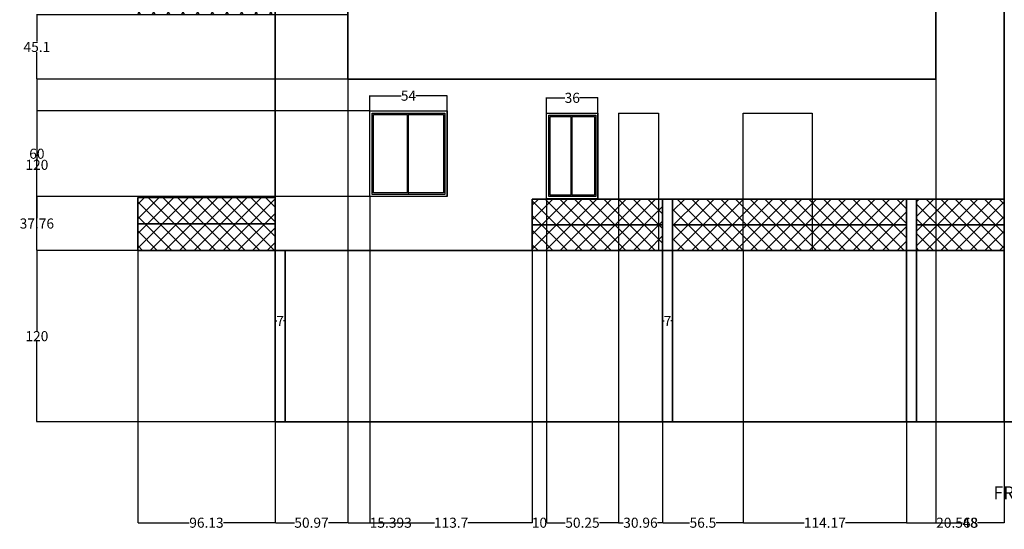
# Model space of a CAD drawing. Units: inches. Extents: x -222 to 1347, y 12 to 1073.
# Tile 1 of 4: x -222 to 467, y 12 to 369. Entities that reach past the tile are written whole.
import ezdxf

# ---------------------------------------------------------------- set-up
doc = ezdxf.new("R2010")
doc.units = ezdxf.units.IN
doc.header["$MEASUREMENT"] = 0
for name, color, linetype, lineweight in [('A-ANNO-DIMS', 2, 'Continuous', 18), ('A-ANNO-TEXT', 7, 'Continuous', 25), ('A-DOOR', 4, 'Continuous', 25), ('A-ELEV', 7, 'Continuous', 35), ('A-ELEV-PATT', 8, 'Continuous', 13), ('A-GLAZ', 4, 'Continuous', 25)]:
    doc.layers.add(name, color=color, linetype=linetype, lineweight=lineweight)
doc.styles.get("Standard").update_dxf_attribs({"font": 'arial.ttf'})
doc.dimstyles.get("Standard").update_dxf_attribs({"dimtxt": 7.0625, "dimasz": 0.18, "dimexe": 0.18, "dimexo": 0.0625, "dimgap": 0.09, "dimtad": 0, "dimtih": 1, "dimtoh": 1, "dimdec": 4, "dimzin": 0, "dimdsep": 46, "dimlunit": 4, "dimtxsty": 'Standard', "dimcen": 0.09, "dimadec": 0, "dimazin": 0, "dimtfac": 1, "dimtdec": 4, "dimtofl": 0, "dimtmove": 0, "dimatfit": 3, "dimfxl": 1, "dimtolj": 1, "dimtzin": 0, "dimarcsym": 0})

# ---------------------------------------------------------------- blocks, each defined once
blk = doc.blocks.new('*U2')
for p, q in [((1.5, 1.5), (1.5, 58.5)), ((1.5, 58.5), (27, 58.5)), ((27, 1.5), (27, 58.5)), ((27, 58.5), (52.5, 58.5)), ((52.5, 58.5), (52.5, 1.5)), ((27, 1.5), (1.5, 1.5)), ((52.5, 1.5), (27, 1.5))]:
    blk.add_line(p, q)
blk.add_lwpolyline([(0, 0), (0, 60), (54, 60), (54, 0)], close=True)
for points in [[(26, 57.5), (26, 2.5), (2.5, 2.5), (2.5, 57.5), (26, 57.5)], [(27, 57.5), (51.5, 57.5), (51.5, 2.5), (27, 2.5)]]:
    blk.add_lwpolyline(points)
blk = doc.blocks.new('*U3')
for p, q in [((1.5, 1.5), (1.5, 58.5)), ((1.5, 58.5), (18, 58.5)), ((18, 1.5), (18, 58.5)), ((18, 58.5), (34.5, 58.5)), ((34.5, 58.5), (34.5, 1.5)), ((18, 1.5), (1.5, 1.5)), ((34.5, 1.5), (18, 1.5))]:
    blk.add_line(p, q)
blk.add_lwpolyline([(0, 0), (0, 60), (36, 60), (36, 0)], close=True)
for points in [[(17, 57.5), (17, 2.5), (2.5, 2.5), (2.5, 57.5), (17, 57.5)], [(18, 57.5), (33.5, 57.5), (33.5, 2.5), (18, 2.5)]]:
    blk.add_lwpolyline(points)
blk = doc.blocks.new('DOOR-700')
for p, q in [((0, 96.26), (0, 0)), ((0, 96.26), (23.43, 96.26)), ((23.43, 96.26), (28.14, 96.26)), ((28.14, 96.26), (28.14, 0))]:
    blk.add_line(p, q)
blk = doc.blocks.new('DOOR-1200')
for p, q in [((0, 0), (0, 96.26)), ((0, 96.26), (48.21, 96.26)), ((48.21, 96.26), (48.21, 0))]:
    blk.add_line(p, q)
blk = doc.blocks.new('*D11')
at = {"layer": 'A-ANNO-DIMS', "color": 0, "lineweight": -2, "transparency": 16777216}
for p, q in [((-139.29, 207.6), (-139.29, 16.83)), ((-43.16, 87.6), (-43.16, 16.83)), ((-139.11, 17.01), (-103.23, 17.01)), ((-43.34, 17.01), (-79.22, 17.01))]:
    blk.add_line(p, q, dxfattribs=at)
at = {"layer": 'A-ANNO-DIMS', "color": 0, "transparency": 16777216}
for points in [[(-139.11, 17.04), (-139.11, 16.98), (-139.29, 17.01)], [(-43.34, 17.04), (-43.34, 16.98), (-43.16, 17.01)]]:
    blk.add_solid(points, dxfattribs=at)
at = {"layer": 'Defpoints', "color": 0, "transparency": 16777216}
for p in [(-139.29, 207.66), (-43.16, 87.66), (-43.16, 17.01)]:
    blk.add_point(p, dxfattribs=at)
at = {"layer": 'A-ANNO-DIMS', "color": 0, "transparency": 16777216, "insert": (-91.23, 17.01), "char_height": 7.062, "attachment_point": 5}
blk.add_mtext('\\A1;96.13', dxfattribs=at)
blk = doc.blocks.new('*D12')
at = {"layer": 'A-ANNO-DIMS', "color": 0, "lineweight": -2, "transparency": 16777216}
for p, q in [((7.81, 327.6), (7.81, 16.83)), ((-43.16, 87.6), (-43.16, 16.83)), ((-42.98, 17.01), (-29.68, 17.01)), ((7.63, 17.01), (-5.67, 17.01))]:
    blk.add_line(p, q, dxfattribs=at)
at = {"layer": 'A-ANNO-DIMS', "color": 0, "transparency": 16777216}
for points in [[(-42.98, 17.04), (-42.98, 16.98), (-43.16, 17.01)], [(7.63, 17.04), (7.63, 16.98), (7.81, 17.01)]]:
    blk.add_solid(points, dxfattribs=at)
at = {"layer": 'Defpoints', "color": 0, "transparency": 16777216}
for p in [(7.81, 327.66), (-43.16, 87.66), (7.81, 17.01)]:
    blk.add_point(p, dxfattribs=at)
at = {"layer": 'A-ANNO-DIMS', "color": 0, "transparency": 16777216, "insert": (-17.68, 17.01), "char_height": 7.062, "attachment_point": 5}
blk.add_mtext('\\A1;50.97', dxfattribs=at)
blk = doc.blocks.new('*D13')
at = {"layer": 'A-ANNO-DIMS', "color": 0, "lineweight": -2, "transparency": 16777216}
for p, q in [((7.81, 327.6), (7.81, 16.83)), ((23.2, 245.36), (23.2, 16.83)), ((7.99, 17.01), (23.02, 17.01)), ((23.2, 17.01), (23.38, 17.01))]:
    blk.add_line(p, q, dxfattribs=at)
at = {"layer": 'A-ANNO-DIMS', "color": 0, "transparency": 16777216}
for points in [[(7.99, 17.04), (7.99, 16.98), (7.81, 17.01)], [(23.02, 17.04), (23.02, 16.98), (23.2, 17.01)]]:
    blk.add_solid(points, dxfattribs=at)
at = {"layer": 'Defpoints', "color": 0, "transparency": 16777216}
for p in [(7.81, 327.66), (23.2, 245.43), (23.2, 17.01)]:
    blk.add_point(p, dxfattribs=at)
at = {"layer": 'A-ANNO-DIMS', "color": 0, "transparency": 16777216, "insert": (37.8, 17.01), "char_height": 7.062, "attachment_point": 5}
blk.add_mtext('\\A1;15.393', dxfattribs=at)
blk = doc.blocks.new('*D14')
at = {"layer": 'A-ANNO-DIMS', "color": 0, "lineweight": -2, "transparency": 16777216}
for p, q in [((23.2, 245.36), (23.2, 16.83)), ((136.89, 207.6), (136.89, 16.83)), ((23.38, 17.01), (68.37, 17.01)), ((136.71, 17.01), (91.72, 17.01))]:
    blk.add_line(p, q, dxfattribs=at)
at = {"layer": 'A-ANNO-DIMS', "color": 0, "transparency": 16777216}
for points in [[(23.38, 17.04), (23.38, 16.98), (23.2, 17.01)], [(136.71, 17.04), (136.71, 16.98), (136.89, 17.01)]]:
    blk.add_solid(points, dxfattribs=at)
at = {"layer": 'Defpoints', "color": 0, "transparency": 16777216}
for p in [(23.2, 245.43), (136.89, 207.66), (136.89, 17.01)]:
    blk.add_point(p, dxfattribs=at)
at = {"layer": 'A-ANNO-DIMS', "color": 0, "transparency": 16777216, "insert": (80.04, 17.01), "char_height": 7.062, "attachment_point": 5}
blk.add_mtext('\\A1;113.7', dxfattribs=at)
blk = doc.blocks.new('*D15')
at = {"layer": 'A-ANNO-DIMS', "color": 0, "lineweight": -2, "transparency": 16777216}
for p, q in [((146.891371, 243.863959), (146.891371, 16.834205)), ((136.890751, 207.601705), (136.890751, 16.834205)), ((136.710751, 17.014205), (136.530751, 17.014205)), ((147.071371, 17.014205), (147.251371, 17.014205))]:
    blk.add_line(p, q, dxfattribs=at)
at = {"layer": 'A-ANNO-DIMS', "color": 0, "transparency": 16777216}
for points in [[(136.710751, 17.044205), (136.710751, 16.984205), (136.890751, 17.014205)], [(147.071371, 17.044205), (147.071371, 16.984205), (146.891371, 17.014205)]]:
    blk.add_solid(points, dxfattribs=at)
at = {"layer": 'Defpoints', "color": 0, "transparency": 16777216}
for p in [(146.891371, 243.926459), (136.890751, 207.664205), (146.891371, 17.014205)]:
    blk.add_point(p, dxfattribs=at)
at = {"layer": 'A-ANNO-DIMS', "color": 0, "transparency": 16777216, "insert": (141.891061, 17.014205), "char_height": 7.0625, "attachment_point": 5}
blk.add_mtext('\\A1;10', dxfattribs=at)
blk = doc.blocks.new('*D16')
at = {"layer": 'A-ANNO-DIMS', "color": 0, "lineweight": -2, "transparency": 16777216}
for p, q in [((146.89, 243.86), (146.89, 16.83)), ((197.14, 207.6), (197.14, 16.83)), ((147.07, 17.01), (159.98, 17.01)), ((196.96, 17.01), (184.05, 17.01))]:
    blk.add_line(p, q, dxfattribs=at)
at = {"layer": 'A-ANNO-DIMS', "color": 0, "transparency": 16777216}
for points in [[(147.07, 17.04), (147.07, 16.98), (146.89, 17.01)], [(196.96, 17.04), (196.96, 16.98), (197.14, 17.01)]]:
    blk.add_solid(points, dxfattribs=at)
at = {"layer": 'Defpoints', "color": 0, "transparency": 16777216}
for p in [(146.89, 243.93), (197.14, 207.66), (197.14, 17.01)]:
    blk.add_point(p, dxfattribs=at)
at = {"layer": 'A-ANNO-DIMS', "color": 0, "transparency": 16777216, "insert": (172.02, 17.01), "char_height": 7.062, "attachment_point": 5}
blk.add_mtext('\\A1;50.25', dxfattribs=at)
blk = doc.blocks.new('*D17')
at = {"layer": 'A-ANNO-DIMS', "color": 0, "lineweight": -2, "transparency": 16777216}
for p, q in [((197.14, 207.6), (197.14, 16.83)), ((228.1, 87.6), (228.1, 16.83)), ((197.32, 17.01), (200.62, 17.01)), ((227.92, 17.01), (224.62, 17.01))]:
    blk.add_line(p, q, dxfattribs=at)
at = {"layer": 'A-ANNO-DIMS', "color": 0, "transparency": 16777216}
for points in [[(197.32, 17.04), (197.32, 16.98), (197.14, 17.01)], [(227.92, 17.04), (227.92, 16.98), (228.1, 17.01)]]:
    blk.add_solid(points, dxfattribs=at)
at = {"layer": 'Defpoints', "color": 0, "transparency": 16777216}
for p in [(197.14, 207.66), (228.1, 87.66), (228.1, 17.01)]:
    blk.add_point(p, dxfattribs=at)
at = {"layer": 'A-ANNO-DIMS', "color": 0, "transparency": 16777216, "insert": (212.62, 17.01), "char_height": 7.062, "attachment_point": 5}
blk.add_mtext('\\A1;30.96', dxfattribs=at)
blk = doc.blocks.new('*D18')
at = {"layer": 'A-ANNO-DIMS', "color": 0, "lineweight": -2, "transparency": 16777216}
for p, q in [((284.6, 207.6), (284.6, 16.83)), ((228.1, 87.6), (228.1, 16.83)), ((228.28, 17.01), (247.06, 17.01)), ((284.42, 17.01), (265.64, 17.01))]:
    blk.add_line(p, q, dxfattribs=at)
at = {"layer": 'A-ANNO-DIMS', "color": 0, "transparency": 16777216}
for points in [[(228.28, 17.04), (228.28, 16.98), (228.1, 17.01)], [(284.42, 17.04), (284.42, 16.98), (284.6, 17.01)]]:
    blk.add_solid(points, dxfattribs=at)
at = {"layer": 'Defpoints', "color": 0, "transparency": 16777216}
for p in [(284.6, 207.66), (228.1, 87.66), (284.6, 17.01)]:
    blk.add_point(p, dxfattribs=at)
at = {"layer": 'A-ANNO-DIMS', "color": 0, "transparency": 16777216, "insert": (256.35, 17.01), "char_height": 7.062, "attachment_point": 5}
blk.add_mtext('\\A1;56.5', dxfattribs=at)
blk = doc.blocks.new('*D19')
at = {"layer": 'A-ANNO-DIMS', "color": 0, "lineweight": -2, "transparency": 16777216}
for p, q in [((284.6, 207.6), (284.6, 16.83)), ((398.78, 87.6), (398.78, 16.83)), ((284.78, 17.01), (327.27, 17.01)), ((398.6, 17.01), (356.11, 17.01))]:
    blk.add_line(p, q, dxfattribs=at)
at = {"layer": 'A-ANNO-DIMS', "color": 0, "transparency": 16777216}
for points in [[(284.78, 17.04), (284.78, 16.98), (284.6, 17.01)], [(398.6, 17.04), (398.6, 16.98), (398.78, 17.01)]]:
    blk.add_solid(points, dxfattribs=at)
at = {"layer": 'Defpoints', "color": 0, "transparency": 16777216}
for p in [(284.6, 207.66), (398.78, 87.66), (398.78, 17.01)]:
    blk.add_point(p, dxfattribs=at)
at = {"layer": 'A-ANNO-DIMS', "color": 0, "transparency": 16777216, "insert": (341.69, 17.01), "char_height": 7.062, "attachment_point": 5}
blk.add_mtext('\\A1;114.17', dxfattribs=at)
blk = doc.blocks.new('*D20')
at = {"layer": 'A-ANNO-DIMS', "color": 0, "lineweight": -2, "transparency": 16777216}
for p, q in [((419.34, 327.6), (419.34, 16.83)), ((398.78, 87.6), (398.78, 16.83)), ((398.96, 17.01), (419.16, 17.01)), ((419.34, 17.01), (419.52, 17.01))]:
    blk.add_line(p, q, dxfattribs=at)
at = {"layer": 'A-ANNO-DIMS', "color": 0, "transparency": 16777216}
for points in [[(398.96, 17.04), (398.96, 16.98), (398.78, 17.01)], [(419.16, 17.04), (419.16, 16.98), (419.34, 17.01)]]:
    blk.add_solid(points, dxfattribs=at)
at = {"layer": 'Defpoints', "color": 0, "transparency": 16777216}
for p in [(419.34, 327.66), (398.78, 87.66), (419.34, 17.01)]:
    blk.add_point(p, dxfattribs=at)
at = {"layer": 'A-ANNO-DIMS', "color": 0, "transparency": 16777216, "insert": (434.34, 17.01), "char_height": 7.062, "attachment_point": 5}
blk.add_mtext('\\A1;20.568', dxfattribs=at)
blk = doc.blocks.new('*D21')
at = {"layer": 'A-ANNO-DIMS', "color": 0, "lineweight": -2, "transparency": 16777216}
for p, q in [((419.34, 327.6), (419.34, 16.83)), ((467.34, 87.6), (467.34, 16.83)), ((419.52, 17.01), (438.05, 17.01)), ((467.16, 17.01), (448.64, 17.01))]:
    blk.add_line(p, q, dxfattribs=at)
at = {"layer": 'A-ANNO-DIMS', "color": 0, "transparency": 16777216}
for points in [[(419.52, 17.04), (419.52, 16.98), (419.34, 17.01)], [(467.16, 17.04), (467.16, 16.98), (467.34, 17.01)]]:
    blk.add_solid(points, dxfattribs=at)
at = {"layer": 'Defpoints', "color": 0, "transparency": 16777216}
for p in [(419.34, 327.66), (467.34, 87.66), (467.34, 17.01)]:
    blk.add_point(p, dxfattribs=at)
at = {"layer": 'A-ANNO-DIMS', "color": 0, "transparency": 16777216, "insert": (443.34, 17.01), "char_height": 7.062, "attachment_point": 5}
blk.add_mtext('\\A1;48', dxfattribs=at)
blk = doc.blocks.new('*D38')
at = {"layer": 'A-ANNO-DIMS', "color": 0, "lineweight": -2, "transparency": 16777216}
for p, q in [((23.2, 245.49), (23.2, 316.26)), ((23.38, 316.08), (45.07, 316.08)), ((77.02, 316.08), (55.33, 316.08)), ((77.2, 245.49), (77.2, 316.26))]:
    blk.add_line(p, q, dxfattribs=at)
at = {"layer": 'A-ANNO-DIMS', "color": 0, "transparency": 16777216}
for points in [[(23.38, 316.11), (23.38, 316.05), (23.2, 316.08)], [(77.02, 316.11), (77.02, 316.05), (77.2, 316.08)]]:
    blk.add_solid(points, dxfattribs=at)
at = {"layer": 'Defpoints', "color": 0, "transparency": 16777216}
for p in [(77.2, 316.08), (23.2, 245.43), (77.2, 245.43)]:
    blk.add_point(p, dxfattribs=at)
at = {"layer": 'A-ANNO-DIMS', "color": 0, "transparency": 16777216, "insert": (50.2, 316.08), "char_height": 7.062, "attachment_point": 5}
blk.add_mtext('\\A1;54', dxfattribs=at)
blk = doc.blocks.new('*D39')
at = {"layer": 'A-ANNO-DIMS', "color": 0, "lineweight": -2, "transparency": 16777216}
for p, q in [((146.89, 243.99), (146.89, 314.76)), ((147.07, 314.58), (159.75, 314.58)), ((182.71, 314.58), (170.03, 314.58)), ((182.89, 243.99), (182.89, 314.76))]:
    blk.add_line(p, q, dxfattribs=at)
at = {"layer": 'A-ANNO-DIMS', "color": 0, "transparency": 16777216}
for points in [[(147.07, 314.61), (147.07, 314.55), (146.89, 314.58)], [(182.71, 314.61), (182.71, 314.55), (182.89, 314.58)]]:
    blk.add_solid(points, dxfattribs=at)
at = {"layer": 'Defpoints', "color": 0, "transparency": 16777216}
for p in [(182.89, 314.58), (146.89, 243.93), (182.89, 243.93)]:
    blk.add_point(p, dxfattribs=at)
at = {"layer": 'A-ANNO-DIMS', "color": 0, "transparency": 16777216, "insert": (164.89, 314.58), "char_height": 7.062, "attachment_point": 5}
blk.add_mtext('\\A1;36', dxfattribs=at)
blk = doc.blocks.new('*D40')
at = {"layer": 'A-ANNO-DIMS', "color": 0, "lineweight": -2, "transparency": 16777216}
for p, q in [((-43.22, 207.66), (-210.12, 207.66)), ((-209.94, 207.48), (-209.94, 151.36)), ((-209.94, 87.84), (-209.94, 143.97)), ((-43.22, 87.66), (-210.12, 87.66))]:
    blk.add_line(p, q, dxfattribs=at)
at = {"layer": 'A-ANNO-DIMS', "color": 0, "transparency": 16777216}
for points in [[(-209.97, 207.48), (-209.91, 207.48), (-209.94, 207.66)], [(-209.97, 87.84), (-209.91, 87.84), (-209.94, 87.66)]]:
    blk.add_solid(points, dxfattribs=at)
at = {"layer": 'Defpoints', "color": 0, "transparency": 16777216}
for p in [(-209.94, 207.66), (-43.16, 207.66), (-43.16, 87.66)]:
    blk.add_point(p, dxfattribs=at)
at = {"layer": 'A-ANNO-DIMS', "color": 0, "transparency": 16777216, "insert": (-209.94, 147.66), "char_height": 7.062, "attachment_point": 5}
blk.add_mtext('\\A1;120', dxfattribs=at)
blk = doc.blocks.new('*D41')
at = {"layer": 'A-ANNO-DIMS', "color": 0, "lineweight": -2, "transparency": 16777216}
for p, q in [((7.74, 327.66), (-210.12, 327.66)), ((-209.94, 327.48), (-209.94, 271.36)), ((-209.94, 207.84), (-209.94, 263.97)), ((-43.22, 207.66), (-210.12, 207.66))]:
    blk.add_line(p, q, dxfattribs=at)
at = {"layer": 'A-ANNO-DIMS', "color": 0, "transparency": 16777216}
for points in [[(-209.97, 327.48), (-209.91, 327.48), (-209.94, 327.66)], [(-209.97, 207.84), (-209.91, 207.84), (-209.94, 207.66)]]:
    blk.add_solid(points, dxfattribs=at)
at = {"layer": 'Defpoints', "color": 0, "transparency": 16777216}
for p in [(-209.94, 327.66), (7.81, 327.66), (-43.16, 207.66)]:
    blk.add_point(p, dxfattribs=at)
at = {"layer": 'A-ANNO-DIMS', "color": 0, "transparency": 16777216, "insert": (-209.94, 267.66), "char_height": 7.062, "attachment_point": 5}
blk.add_mtext('\\A1;120', dxfattribs=at)
blk = doc.blocks.new('*D42')
at = {"layer": 'A-ANNO-DIMS', "color": 0, "lineweight": -2, "transparency": 16777216}
for p, q in [((7.74, 372.77), (-210.12, 372.77)), ((-209.94, 372.59), (-209.94, 353.91)), ((-209.94, 327.84), (-209.94, 346.52)), ((7.74, 327.66), (-210.12, 327.66))]:
    blk.add_line(p, q, dxfattribs=at)
at = {"layer": 'A-ANNO-DIMS', "color": 0, "transparency": 16777216}
for points in [[(-209.97, 372.59), (-209.91, 372.59), (-209.94, 372.77)], [(-209.97, 327.84), (-209.91, 327.84), (-209.94, 327.66)]]:
    blk.add_solid(points, dxfattribs=at)
at = {"layer": 'Defpoints', "color": 0, "transparency": 16777216}
for p in [(-209.94, 372.77), (7.81, 372.77), (7.81, 327.66)]:
    blk.add_point(p, dxfattribs=at)
at = {"layer": 'A-ANNO-DIMS', "color": 0, "transparency": 16777216, "insert": (-209.94, 350.21), "char_height": 7.062, "attachment_point": 5}
blk.add_mtext('\\A1;45.1', dxfattribs=at)
blk = doc.blocks.new('*D48')
at = {"layer": 'A-ANNO-DIMS', "color": 0, "lineweight": -2, "transparency": 16777216}
for p, q in [((23.14, 245.43), (-210.12, 245.43)), ((-209.94, 245.25), (-209.94, 230.24)), ((-209.94, 207.84), (-209.94, 222.85)), ((136.83, 207.66), (-210.12, 207.66))]:
    blk.add_line(p, q, dxfattribs=at)
at = {"layer": 'A-ANNO-DIMS', "color": 0, "transparency": 16777216}
for points in [[(-209.97, 245.25), (-209.91, 245.25), (-209.94, 245.43)], [(-209.97, 207.84), (-209.91, 207.84), (-209.94, 207.66)]]:
    blk.add_solid(points, dxfattribs=at)
at = {"layer": 'Defpoints', "color": 0, "transparency": 16777216}
for p in [(-209.94, 245.43), (23.2, 245.43), (136.89, 207.66)]:
    blk.add_point(p, dxfattribs=at)
at = {"layer": 'A-ANNO-DIMS', "color": 0, "transparency": 16777216, "insert": (-209.94, 226.55), "char_height": 7.062, "attachment_point": 5}
blk.add_mtext('\\A1;37.76', dxfattribs=at)
blk = doc.blocks.new('*D49')
at = {"layer": 'A-ANNO-DIMS', "color": 0, "lineweight": -2, "transparency": 16777216}
for p, q in [((23.14, 305.43), (-210.12, 305.43)), ((-209.94, 305.25), (-209.94, 279.12)), ((-209.94, 245.61), (-209.94, 271.73)), ((23.14, 245.43), (-210.12, 245.43))]:
    blk.add_line(p, q, dxfattribs=at)
at = {"layer": 'A-ANNO-DIMS', "color": 0, "transparency": 16777216}
for points in [[(-209.97, 305.25), (-209.91, 305.25), (-209.94, 305.43)], [(-209.97, 245.61), (-209.91, 245.61), (-209.94, 245.43)]]:
    blk.add_solid(points, dxfattribs=at)
at = {"layer": 'Defpoints', "color": 0, "transparency": 16777216}
for p in [(-209.94, 305.43), (23.2, 305.43), (23.2, 245.43)]:
    blk.add_point(p, dxfattribs=at)
at = {"layer": 'A-ANNO-DIMS', "color": 0, "transparency": 16777216, "insert": (-209.94, 275.43), "char_height": 7.062, "attachment_point": 5}
blk.add_mtext('\\A1;60', dxfattribs=at)
blk = doc.blocks.new('*D76')
at = {"layer": 'A-ANNO-DIMS', "color": 0, "lineweight": -2, "transparency": 16777216}
for p, q in [((228.1, 87.73), (228.1, 158.49)), ((228.28, 158.31), (229.22, 158.31)), ((234.92, 158.31), (233.98, 158.31)), ((235.1, 87.73), (235.1, 158.49))]:
    blk.add_line(p, q, dxfattribs=at)
at = {"layer": 'A-ANNO-DIMS', "color": 0, "transparency": 16777216}
for points in [[(228.28, 158.34), (228.28, 158.28), (228.1, 158.31)], [(234.92, 158.34), (234.92, 158.28), (235.1, 158.31)]]:
    blk.add_solid(points, dxfattribs=at)
at = {"layer": 'Defpoints', "color": 0, "transparency": 16777216}
for p in [(235.1, 158.31), (228.1, 87.66), (235.1, 87.66)]:
    blk.add_point(p, dxfattribs=at)
at = {"layer": 'A-ANNO-DIMS', "color": 0, "transparency": 16777216, "insert": (231.6, 158.31), "char_height": 7.062, "attachment_point": 5}
blk.add_mtext('\\A1;7', dxfattribs=at)
blk = doc.blocks.new('*D77')
at = {"layer": 'A-ANNO-DIMS', "color": 0, "lineweight": -2, "transparency": 16777216}
for p, q in [((-43.16, 87.73), (-43.16, 158.49)), ((-42.98, 158.31), (-42.04, 158.31)), ((-36.34, 158.31), (-37.28, 158.31)), ((-36.16, 87.73), (-36.16, 158.49))]:
    blk.add_line(p, q, dxfattribs=at)
at = {"layer": 'A-ANNO-DIMS', "color": 0, "transparency": 16777216}
for points in [[(-42.98, 158.34), (-42.98, 158.28), (-43.16, 158.31)], [(-36.34, 158.34), (-36.34, 158.28), (-36.16, 158.31)]]:
    blk.add_solid(points, dxfattribs=at)
at = {"layer": 'Defpoints', "color": 0, "transparency": 16777216}
for p in [(-36.16, 158.31), (-43.16, 87.66), (-36.16, 87.66)]:
    blk.add_point(p, dxfattribs=at)
at = {"layer": 'A-ANNO-DIMS', "color": 0, "transparency": 16777216, "insert": (-39.66, 158.31), "char_height": 7.062, "attachment_point": 5}
blk.add_mtext('\\A1;7', dxfattribs=at)

msp = doc.modelspace()

# ---------------------------------------------------------------- hatches: boundary and pattern name
at = {"layer": 'A-ELEV-PATT'}
h = msp.add_hatch(dxfattribs=at)
h.set_pattern_fill('ANSI37', color=256, scale=58)
h.paths.add_polyline_path([(-43.1601, 648.7576), (-139.2916, 648.7576), (-139.2916, 630.2077), (-43.1601, 630.2077)])
h.paths.add_polyline_path([(-43.1601, 630.2077), (-139.2916, 630.2077), (-139.2916, 611.6578), (-43.1601, 611.6578)])
h.paths.add_polyline_path([(-43.1601, 529.8651), (-139.2916, 529.8651), (-139.2916, 511.3152), (-43.1601, 511.3152)])
h.paths.add_polyline_path([(-43.1601, 511.3152), (-139.2916, 511.3152), (-139.2916, 492.7653), (-43.1601, 492.7653)])
h.paths.add_polyline_path([(-43.1601, 409.8651), (-139.2916, 409.8651), (-139.2916, 391.3152), (-43.1601, 391.3152)])
h.paths.add_polyline_path([(-43.1601, 391.3152), (-139.2916, 391.3152), (-139.2916, 372.7653), (-43.1601, 372.7653)])
h.paths.add_polyline_path([(-43.1601, 244.764), (-139.2916, 244.764), (-139.2916, 226.2141), (-43.1601, 226.2141)])
h.paths.add_polyline_path([(-43.1601, 226.2141), (-139.2916, 226.2141), (-139.2916, 207.6642), (-43.1601, 207.6642)])
h = msp.add_hatch(dxfattribs=at)
h.set_pattern_fill('ANSI37', color=256, scale=58)
h.paths.add_polyline_path([(197.1405, 243.6642), (136.8908, 243.6642), (136.8908, 225.6642), (197.1405, 225.6642)])
h.paths.add_polyline_path([(197.1405, 225.6642), (136.8908, 225.6642), (136.8908, 207.6642), (197.1405, 207.6642)])
h.paths.add_polyline_path([(225.2842, 243.6642), (197.1405, 243.6642), (197.1405, 225.6642), (225.2842, 225.6642)])
h.paths.add_polyline_path([(225.2842, 225.6642), (197.1405, 225.6642), (197.1405, 207.6642), (225.2842, 207.6642)])
h.paths.add_polyline_path([(228.1006, 243.6642), (225.2842, 243.6642), (225.2842, 225.6642), (228.1006, 225.6642)])
h.paths.add_polyline_path([(228.1006, 225.6642), (225.2842, 225.6642), (225.2842, 207.6642), (228.1006, 207.6642)])
h.paths.add_polyline_path([(284.6018, 243.6642), (235.1006, 243.6642), (235.1006, 225.6642), (284.6018, 225.6642)])
h.paths.add_polyline_path([(284.6018, 225.6642), (235.1006, 225.6642), (235.1006, 207.6642), (284.6018, 207.6642)])
h.paths.add_polyline_path([(332.8148, 243.6642), (284.6018, 243.6642), (284.6018, 225.6642), (332.8148, 225.6642)])
h.paths.add_polyline_path([(332.8148, 225.6642), (284.6018, 225.6642), (284.6018, 207.6642), (332.8148, 207.6642)])
h.paths.add_polyline_path([(398.776, 243.6642), (332.8148, 243.6642), (332.8148, 225.6642), (398.776, 225.6642)])
h.paths.add_polyline_path([(398.776, 225.6642), (332.8148, 225.6642), (332.8148, 207.6642), (398.776, 207.6642)])
h.paths.add_polyline_path([(467.3436, 243.6642), (405.776, 243.6642), (405.776, 225.6642), (467.3436, 225.6642)])
h.paths.add_polyline_path([(467.3436, 225.6642), (405.776, 225.6642), (405.776, 207.6642), (467.3436, 207.6642)])

# ---------------------------------------------------------------- linework, layer by layer
at = {"layer": 'A-ELEV'}
for p, q in [((-43.1601, 207.6642), (-43.1601, 780.7653)), ((467.3436, 87.6642), (467.3436, 780.7653)), ((7.8066, 584.7569), (7.8066, 347.9663)), ((419.3436, 447.6642), (419.3436, 327.6642)), ((7.8066, 327.6642), (7.8066, 347.9663)), ((7.8066, 327.6642), (408.7725, 327.6642)), ((419.3436, 327.6642), (408.7725, 327.6642)), ((-43.1601, 244.764), (-139.2916, 244.764)), ((-139.2916, 244.764), (-139.2916, 207.6642)), ((228.1006, 243.6642), (136.8908, 243.6642)), ((136.8908, 243.6642), (136.8908, 207.6642)), ((228.1006, 207.6642), (228.1006, 243.6642)), ((228.1006, 243.6642), (235.1006, 243.6642)), ((235.1006, 243.6642), (235.1006, 207.6642)), ((235.1006, 243.6642), (398.776, 243.6642)), ((398.776, 243.6642), (398.776, 207.6642)), ((398.776, 243.6642), (405.776, 243.6642)), ((405.776, 243.6642), (405.776, 207.6642)), ((405.776, 243.6642), (467.3436, 243.6642)), ((-139.2916, 226.2141), (-43.1601, 226.2141)), ((136.8908, 225.6642), (228.1006, 225.6642)), ((235.1006, 225.6642), (398.776, 225.6642)), ((405.776, 225.6642), (467.3436, 225.6642)), ((-43.1601, 207.6642), (-139.2916, 207.6642)), ((-43.1601, 87.6642), (-43.1601, 207.6642)), ((-43.1601, 207.6642), (467.3436, 207.6642)), ((-36.1601, 87.6642), (-36.1601, 207.6642)), ((228.1006, 87.6642), (228.1006, 207.6642)), ((235.1006, 87.6642), (235.1006, 207.6642)), ((398.776, 87.6642), (398.776, 207.6642)), ((405.776, 87.6642), (405.776, 207.6642)), ((40.3442, 87.6642), (-43.1601, 87.6642)), ((40.3442, 87.6642), (971.5102, 87.6642))]:
    msp.add_line(p, q, dxfattribs=at)

# ---------------------------------------------------------------- block references
at = {"layer": 'A-DOOR'}
for name, p in [('DOOR-700', (197.14, 207.664)), ('DOOR-1200', (284.602, 207.664))]:
    msp.add_blockref(name, p, dxfattribs=at)
at = {"layer": 'A-GLAZ'}
for name, p in [('*U2', (23.1991, 245.4265)), ('*U3', (146.8914, 243.9265))]:
    msp.add_blockref(name, p, dxfattribs=at)

# ---------------------------------------------------------------- texts
at = {"layer": 'A-ANNO-TEXT', "insert": (459.7334, 42.4682), "char_height": 9, "attachment_point": 1}
msp.add_mtext_dynamic_manual_height_columns('FRONT ELEVATION', width=262.403547, gutter_width=1, heights=[0], dxfattribs=at)

# ---------------------------------------------------------------- dimensions: what is measured, and where the dimension line sits
at = {"layer": 'A-ANNO-DIMS'}
for base, p1, p2, override, picture, middle in [((-209.9416, 372.7653), (7.8066, 327.6642), (7.8066, 372.7653), {"dimdec": 1, "dimlfac": 1, "dimrnd": 0, "dimzin": 0, "dimdsep": 46, "dimlunit": 2}, '*D42', (-209.9416, 350.2148)), ((-209.9416, 327.6642), (-43.1601, 207.6642), (7.8066, 327.6642), {"dimdec": 0, "dimlfac": 1, "dimrnd": 0, "dimzin": 0, "dimdsep": 46, "dimlunit": 2}, '*D41', (-209.9416, 267.6642)), ((-209.9416, 305.4265), (23.1991, 245.4265), (23.1991, 305.4265), {"dimdec": 0, "dimlfac": 1, "dimrnd": 0, "dimzin": 0, "dimdsep": 46, "dimlunit": 2}, '*D49', (-209.9416, 275.4265)), ((-209.9416, 245.4265), (136.8908, 207.6642), (23.1991, 245.4265), {"dimdec": 2, "dimlfac": 1, "dimrnd": 0, "dimzin": 0, "dimdsep": 46, "dimlunit": 2}, '*D48', (-209.9416, 226.5453)), ((-209.9416, 207.6642), (-43.1601, 87.6642), (-43.1601, 207.6642), {"dimdec": 0, "dimlfac": 1, "dimrnd": 0, "dimzin": 0, "dimdsep": 46, "dimlunit": 2}, '*D40', (-209.9416, 147.6642))]:
    dim = msp.add_linear_dim(base=base, p1=p1, p2=p2, angle=90, dimstyle='Standard', override=override, dxfattribs=at)
    dim.commit()
    dim.dimension.update_dxf_attribs({"geometry": picture, "text_midpoint": middle})
for base, p1, p2, override, picture, middle in [((7.8066, 17.0142), (-43.1601, 87.6642), (7.8066, 327.6642), {"dimdec": 2, "dimlfac": 1, "dimrnd": 0, "dimzin": 0, "dimdsep": 46, "dimlunit": 2}, '*D12', (-17.6768, 17.0142)), ((23.19912, 17.01421), (7.80659, 327.6642), (23.19912, 245.42646), {"dimdec": 3, "dimlfac": 1, "dimrnd": 0, "dimzin": 0, "dimdsep": 46, "dimlunit": 2}, '*D13', (37.79645, 17.01421)), ((419.3436, 17.0142), (398.776, 87.6642), (419.3436, 327.6642), {"dimdec": 3, "dimlfac": 1, "dimrnd": 0, "dimzin": 0, "dimdsep": 46, "dimlunit": 2}, '*D20', (434.3408, 17.0142)), ((467.3436, 17.0142), (419.3436, 327.6642), (467.3436, 87.6642), {"dimdec": 0, "dimlfac": 1, "dimrnd": 0, "dimzin": 0, "dimdsep": 46, "dimlunit": 2}, '*D21', (443.3436, 17.0142)), ((77.1991, 316.0765), (23.1991, 245.4265), (77.1991, 245.4265), {"dimdec": 0, "dimlfac": 1, "dimrnd": 0, "dimzin": 0, "dimdsep": 46, "dimlunit": 2}, '*D38', (50.1991, 316.0765)), ((182.8914, 314.5765), (146.8914, 243.9265), (182.8914, 243.9265), {"dimdec": 0, "dimlfac": 1, "dimrnd": 0, "dimzin": 0, "dimdsep": 46, "dimlunit": 2}, '*D39', (164.8914, 314.5765)), ((136.8908, 17.0142), (23.1991, 245.4265), (136.8908, 207.6642), {"dimdec": 1, "dimlfac": 1, "dimrnd": 0, "dimzin": 0, "dimdsep": 46, "dimlunit": 2}, '*D14', (80.0449, 17.0142)), ((146.8914, 17.0142), (136.8908, 207.6642), (146.8914, 243.9265), {"dimdec": 0, "dimlfac": 1, "dimrnd": 0, "dimzin": 0, "dimdsep": 46, "dimlunit": 2}, '*D15', (141.8911, 17.0142)), ((197.1405, 17.0142), (146.8914, 243.9265), (197.1405, 207.6642), {"dimdec": 2, "dimlfac": 1, "dimrnd": 0, "dimzin": 0, "dimdsep": 46, "dimlunit": 2}, '*D16', (172.0159, 17.0142)), ((-43.1601, 17.0142), (-139.2916, 207.6642), (-43.1601, 87.6642), {"dimdec": 2, "dimlfac": 1, "dimrnd": 0, "dimzin": 0, "dimdsep": 46, "dimlunit": 2}, '*D11', (-91.2258, 17.0142)), ((228.1006, 17.0142), (197.1405, 207.6642), (228.1006, 87.6642), {"dimdec": 2, "dimlfac": 1, "dimrnd": 0, "dimzin": 0, "dimdsep": 46, "dimlunit": 2}, '*D17', (212.6205, 17.0142)), ((284.6018, 17.0142), (228.1006, 87.6642), (284.6018, 207.6642), {"dimdec": 1, "dimlfac": 1, "dimrnd": 0, "dimzin": 0, "dimdsep": 46, "dimlunit": 2}, '*D18', (256.3512, 17.0142)), ((398.776, 17.0142), (284.6018, 207.6642), (398.776, 87.6642), {"dimdec": 2, "dimlfac": 1, "dimrnd": 0, "dimzin": 0, "dimdsep": 46, "dimlunit": 2}, '*D19', (341.6889, 17.0142)), ((-36.1601, 158.3142), (-43.1601, 87.6642), (-36.1601, 87.6642), {"dimdec": 0, "dimlfac": 1, "dimrnd": 0, "dimzin": 0, "dimdsep": 46, "dimlunit": 2}, '*D77', (-39.6601, 158.3142)), ((235.1006, 158.3142), (228.1006, 87.6642), (235.1006, 87.6642), {"dimdec": 0, "dimlfac": 1, "dimrnd": 0, "dimzin": 0, "dimdsep": 46, "dimlunit": 2}, '*D76', (231.6006, 158.3142))]:
    dim = msp.add_linear_dim(base=base, p1=p1, p2=p2, dimstyle='Standard', override=override, dxfattribs=at)
    dim.commit()
    dim.dimension.update_dxf_attribs({"geometry": picture, "text_midpoint": middle})

doc.saveas('drawing.dxf')
